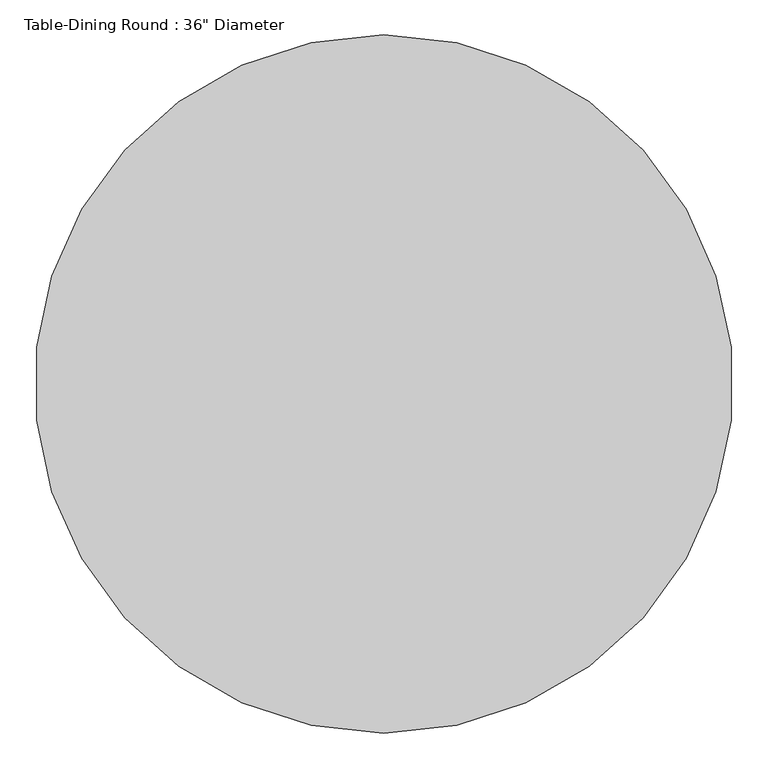
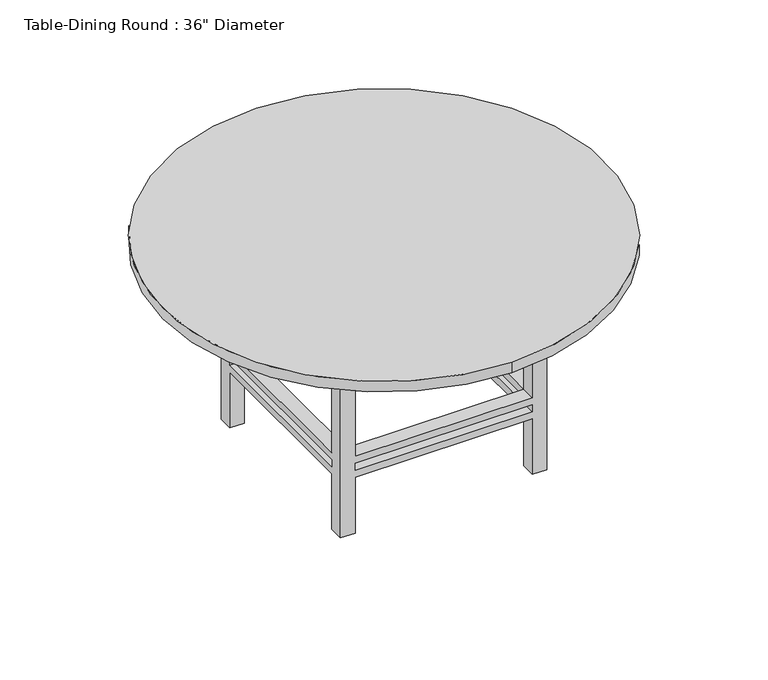
"""IFC4 building model written with IfcOpenShell, lengths in millimetres: furniture geometry."""

from ifc_helpers import new_model, si_unit, point, frame, frame_2d, origin, place, context, project, spatial, polyline, circle_curve, trimmed, segment, composite_curve, outline, extrude, faceted_brep, source, transform, mapped, element, save


def furniture_720490b2(model_context):
    return source(origin(), model_context, "Body", "SolidModel", [
        faceted_brep([(-201.1180328, 170.7213115, 723.9), (-251.9180328, 170.7213115, 723.9), (-251.9180328, 119.9213115, 723.9), (-201.1180328, 119.9213115, 723.9), (408.4819672, 170.7213115, 723.9), (408.4819672, 119.9213115, 723.9), (459.2819672, 119.9213115, 723.9), (459.2819672, 170.7213115, 723.9), (408.4819672, -540.4786885, 723.9), (459.2819672, -540.4786885, 723.9), (459.2819672, -489.6786885, 723.9), (408.4819672, -489.6786885, 723.9), (-201.1180328, -540.4786885, 723.9), (-201.1180328, -489.6786885, 723.9), (-251.9180328, -489.6786885, 723.9), (-251.9180328, -540.4786885, 723.9), (-201.1180328, 170.7213115, 0.0), (-201.1180328, 119.9213115, 0.0), (-251.9180328, 119.9213115, 0.0), (-251.9180328, 170.7213115, 0.0), (408.4819672, 170.7213115, 0.0), (459.2819672, 170.7213115, 0.0), (459.2819672, 119.9213115, 0.0), (408.4819672, 119.9213115, 0.0), (408.4819672, -540.4786885, 0.0), (408.4819672, -489.6786885, 0.0), (459.2819672, -489.6786885, 0.0), (459.2819672, -540.4786885, 0.0), (-201.1180328, -540.4786885, 0.0), (-251.9180328, -540.4786885, 0.0), (-251.9180328, -489.6786885, 0.0), (-201.1180328, -489.6786885, 0.0), (-201.1180328, 170.7213115, 279.4), (408.4819672, 170.7213115, 279.4), (408.4819672, 170.7213115, 203.2), (-201.1180328, 170.7213115, 203.2), (408.4819672, 170.7213115, 228.6), (408.4819672, 170.7213115, 254.0), (-201.1180328, 170.7213115, 254.0), (-201.1180328, 170.7213115, 228.6), (-251.9180328, 119.9213115, 203.2), (-251.9180328, -489.6786885, 203.2), (-251.9180328, -489.6786885, 279.4), (-251.9180328, 119.9213115, 279.4), (-251.9180328, 119.9213115, 228.6), (-251.9180328, 119.9213115, 254.0), (-251.9180328, -489.6786885, 254.0), (-251.9180328, -489.6786885, 228.6), (-201.1180328, 119.9213115, 279.4), (-201.1180328, 119.9213115, 203.2), (-201.1180328, 119.9213115, 228.6), (-201.1180328, 119.9213115, 254.0), (408.4819672, 119.9213115, 279.4), (408.4819672, 119.9213115, 203.2), (408.4819672, 119.9213115, 228.6), (408.4819672, 119.9213115, 254.0), (459.2819672, 119.9213115, 279.4), (459.2819672, 119.9213115, 203.2), (459.2819672, 119.9213115, 228.6), (459.2819672, 119.9213115, 254.0), (459.2819672, -489.6786885, 279.4), (459.2819672, -489.6786885, 203.2), (459.2819672, -489.6786885, 228.6), (459.2819672, -489.6786885, 254.0), (408.4819672, -540.4786885, 279.4), (-201.1180328, -540.4786885, 279.4), (-201.1180328, -540.4786885, 203.2), (408.4819672, -540.4786885, 203.2), (-201.1180328, -540.4786885, 228.6), (-201.1180328, -540.4786885, 254.0), (408.4819672, -540.4786885, 254.0), (408.4819672, -540.4786885, 228.6), (408.4819672, -489.6786885, 279.4), (408.4819672, -489.6786885, 203.2), (408.4819672, -489.6786885, 228.6), (408.4819672, -489.6786885, 254.0), (-201.1180328, -489.6786885, 279.4), (-201.1180328, -489.6786885, 203.2), (-201.1180328, -489.6786885, 228.6), (-201.1180328, -489.6786885, 254.0)], [[[0, 1, 2, 3]], [[4, 5, 6, 7]], [[8, 9, 10, 11]], [[12, 13, 14, 15]], [[16, 17, 18, 19]], [[20, 21, 22, 23]], [[24, 25, 26, 27]], [[28, 29, 30, 31]], [[1, 0, 32, 33, 4, 7, 21, 20, 34, 35, 16, 19], [36, 37, 38, 39]], [[2, 1, 19, 18, 40, 41, 30, 29, 15, 14, 42, 43], [44, 45, 46, 47]], [[3, 2, 43, 48]], [[18, 17, 49, 40]], [[44, 50, 51, 45]], [[0, 3, 48, 32]], [[17, 16, 35, 49]], [[50, 39, 38, 51]], [[5, 4, 33, 52]], [[20, 23, 53, 34]], [[36, 54, 55, 37]], [[6, 5, 52, 56]], [[23, 22, 57, 53]], [[54, 58, 59, 55]], [[21, 7, 6, 56, 60, 10, 9, 27, 26, 61, 57, 22], [62, 63, 59, 58]], [[27, 9, 8, 64, 65, 12, 15, 29, 28, 66, 67, 24], [68, 69, 70, 71]], [[11, 10, 60, 72]], [[26, 25, 73, 61]], [[62, 74, 75, 63]], [[8, 11, 72, 64]], [[25, 24, 67, 73]], [[74, 71, 70, 75]], [[13, 12, 65, 76]], [[28, 31, 77, 66]], [[68, 78, 79, 69]], [[14, 13, 76, 42]], [[31, 30, 41, 77]], [[78, 47, 46, 79]], [[54, 74, 62, 58]], [[74, 78, 68, 71]], [[78, 50, 44, 47]], [[50, 54, 36, 39]], [[53, 49, 35, 34]], [[49, 77, 41, 40]], [[77, 73, 67, 66]], [[73, 53, 57, 61]], [[74, 54, 53, 73]], [[78, 74, 73, 77]], [[50, 78, 77, 49]], [[54, 50, 49, 53]], [[52, 72, 60, 56]], [[72, 76, 65, 64]], [[76, 48, 43, 42]], [[48, 52, 33, 32]], [[55, 51, 38, 37]], [[51, 79, 46, 45]], [[79, 75, 70, 69]], [[75, 55, 59, 63]], [[72, 52, 55, 75]], [[76, 72, 75, 79]], [[48, 76, 79, 51]], [[52, 48, 51, 55]]]),
        extrude(outline(polyline([(484.6819672, 196.1213115), (484.6819672, -565.8786885), (-277.3180328, -565.8786885), (-277.3180328, 196.1213115), (484.6819672, 196.1213115)]), holes=[polyline([(459.2819672, 170.7213115), (-251.9180328, 170.7213115), (-251.9180328, -540.4786885), (459.2819672, -540.4786885), (459.2819672, 170.7213115)])]), frame((0.0, 0.0, 647.7), z_axis=(0.0, 0.0, 1.0), x_axis=(1.0, 0.0, 0.0)), (0.0, 0.0, 1.0), 76.2),
        extrude(outline(composite_curve([segment(trimmed(circle_curve(frame_2d((103.6819672, -184.8786885)), 762.0), [point((103.6819672, -946.8786885))], [point((103.6819672, 577.1213115))], False, "CARTESIAN"), True, "CONTINUOUS"), segment(trimmed(circle_curve(frame_2d((103.6819672, -184.8786885)), 762.0), [point((103.6819672, 577.1213115))], [point((103.6819672, -946.8786885))], False, "CARTESIAN"), True, "CONTINUOUS")], self_intersect=False)), frame((0.0, 0.0, 723.9), z_axis=(0.0, 0.0, 1.0), x_axis=(1.0, 0.0, 0.0)), (0.0, 0.0, 1.0), 38.1),
    ])


if __name__ == "__main__":
    model = new_model("IFC4")
    model_context = context("Model", 3, world=origin())
    ifc_project = project(units=[si_unit("LENGTHUNIT", "METRE", prefix="MILLI")], contexts=[model_context])
    site = spatial("IfcSite", under=ifc_project)
    building = spatial("IfcBuilding", under=site)
    placement = place(None, origin())
    furniture_shape = furniture_720490b2(model_context)
    element("IfcFurniture", 1, ObjectType="Table-Dining Round : 36\" Diameter", at=placement, inside=building, context=model_context, shape_type="MappedRepresentation", body=[
        mapped(furniture_shape, transform((0.0, 0.0, 0.0), x_axis=(1.0, 0.0, 0.0), y_axis=(0.0, 1.0, 0.0), z_axis=(0.0, 0.0, 1.0))),
    ])
    save(model, "model.ifc")

# Revit data of these elements
# Type "Table-Dining Round : 36\" Diameter"
#   Assembly Code = "E2020200"
#   Diameter = 5' - 0"
#   Height = 2' - 6"
#   Base Material = Pine
#   Top Material = Laminate, Linen, Matte
#   Default Elevation = 0
# Element 1 (IfcFurniture, "Table-Dining Round : 36\" Diameter")
#   Materials on its faces: "Pine", "Laminate, Linen, Matte"
# Materials
#   "Pine": class "Wood", colour RGB 223 192 134, transparency 0, Description = "Pinus Echinata", Cost = 0
#   "Laminate, Linen, Matte": class "Plastic", colour RGB 249 239 230, transparency 0, Description = "Plastic Laminate - Linen, Matte", Cost = 0
